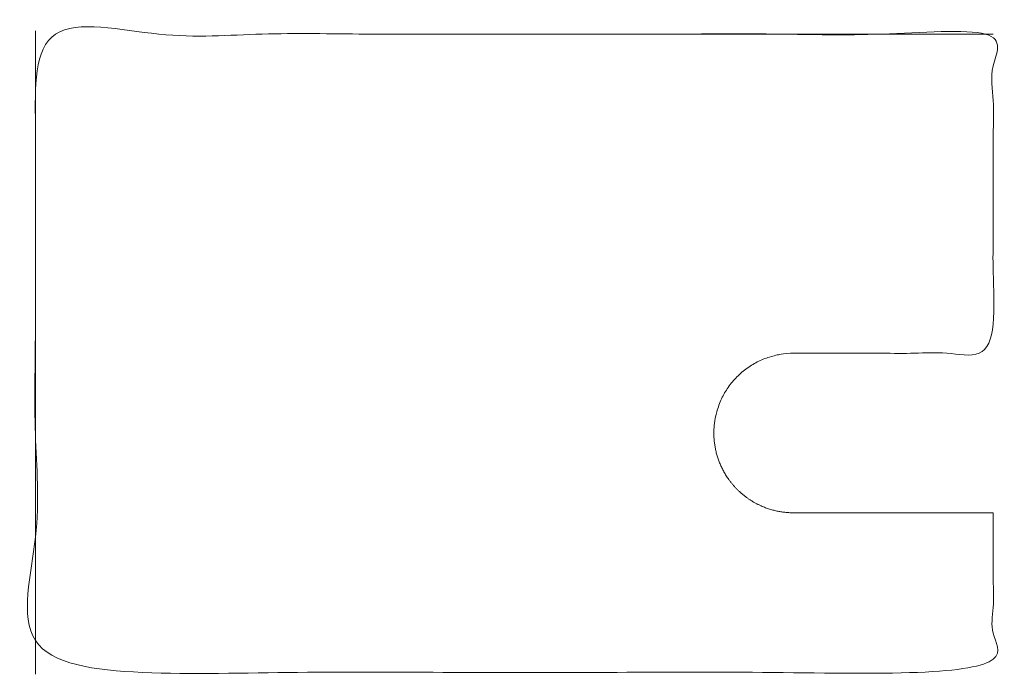
# Model space of a CAD drawing. Units: millimetres. Extents: x 36.9 to 135.6, y 125.6 to 191.5.
import ezdxf

# ---------------------------------------------------------------- set-up
doc = ezdxf.new("R2010")
doc.units = ezdxf.units.MM
doc.layers.add('M-CONS', color=8, linetype='Continuous', lineweight=18)

msp = doc.modelspace()

# ---------------------------------------------------------------- linework, layer by layer
at = {"layer": 'M-CONS', "extrusion": (0, 1, 0), "elevation": 190.007}
msp.add_lwpolyline([(-94.479, 16), (-134.48, 16), (-94.479, 44)], close=True, dxfattribs=at)
at = {"layer": 'M-CONS'}
msp.add_rational_spline([(134.48, 142.007), (124.48, 142.007), (114.48, 142.007), (106.48, 142.007), (106.48, 150.007), (106.48, 158.007), (114.48, 158.007), (124.48, 158.007), (134.48, 158.007), (134.48, 174.007), (134.48, 190.007), (86.48, 190.007), (38.48, 190.007), (38.48, 158.007), (38.48, 126.007), (86.48, 126.007), (134.48, 126.007), (134.48, 134.007), (134.48, 142.007)], [1, 1, 1, 0.707106781187, 1, 0.707106781187, 1, 1, 1, 1, 1, 1, 1, 1, 1, 1, 1, 1, 1], degree=2, knots=[0, 0, 0, 1, 1, 2.570796, 2.570796, 4.141593, 4.141593, 5.141593, 5.141593, 6.141593, 6.141593, 7.141593, 7.141593, 8.141593, 8.141593, 9.141593, 9.141593, 10.141593, 10.141593, 10.141593], dxfattribs=at)
at = {"layer": 'M-CONS', "extrusion": (1, 0, 1e-16)}
msp.add_rational_spline([(38.48, 126.007, 16), (38.48, 126.007, 8), (38.48, 126.007), (38.48, 158.007), (38.48, 190.007), (38.48, 190.007, 32), (38.48, 190.007, 64), (38.48, 165.736, 72.63), (38.48, 145.127, 57.174), (38.48, 124.519, 41.717), (38.48, 126.007, 16)], [1, 1, 1, 1, 1, 1, 1, 0.881127345618, 1, 0.881127345618, 1], degree=2, knots=[0, 0, 0, 1, 1, 2, 2, 3, 3, 3.985111, 3.985111, 4.970222, 4.970222, 4.970222], dxfattribs=at)

doc.saveas('drawing.dxf')
